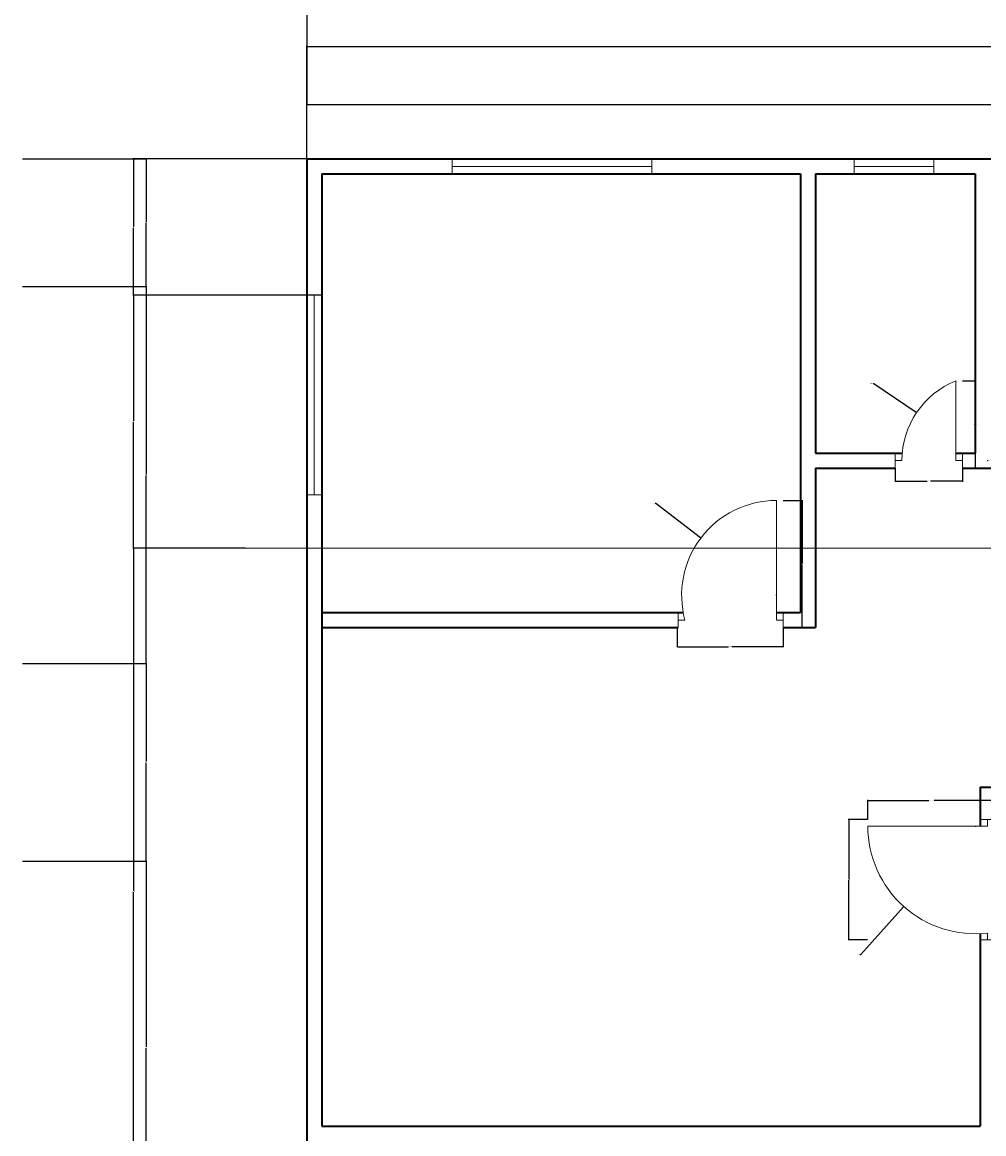
# Model space of a CAD drawing. Units: inches. Extents: x 992 to 2287, y 1476 to 2866.
# Tile 6 of 9: x 1531 to 1821, y 1987 to 2321. Entities that reach past the tile are written whole.
import ezdxf

# ---------------------------------------------------------------- set-up
doc = ezdxf.new("R2010")
doc.units = ezdxf.units.IN
for name, color, linetype, lineweight in [('A-ANNO-DIMS', 2, 'Continuous', 18), ('A-ANNO-SYMB', 2, 'Continuous', 18), ('A-DOOR', 3, 'Continuous', 18), ('A-GLAZ', 4, 'Continuous', 18), ('A-WALL', 7, 'Continuous', 35)]:
    doc.layers.add(name, color=color, linetype=linetype, lineweight=lineweight)
doc.styles.get("Standard").update_dxf_attribs({"font": 'arial.ttf'})
doc.dimstyles.get("Standard").update_dxf_attribs({"dimtxt": 0.18, "dimasz": 0.18, "dimexe": 0.18, "dimexo": 0.0625, "dimgap": 0.09, "dimtad": 0, "dimtih": 1, "dimtoh": 1, "dimdec": 4, "dimzin": 0, "dimdsep": 46, "dimtxsty": 'Standard', "dimcen": 0.09, "dimadec": 0, "dimazin": 0, "dimtfac": 1, "dimtdec": 4, "dimtofl": 0, "dimtmove": 0, "dimatfit": 3, "dimfxl": 1, "dimtolj": 1, "dimtzin": 0, "dimarcsym": 0})

# ---------------------------------------------------------------- blocks, each defined once
blk = doc.blocks.new('DOOR-SINGLE-36IN-01')
for p, q in [((36, 34.15), (0, 34.15)), ((38.25, 36.15), (33.75, 36.15)), ((33.75, 36.15), (36, 36.15)), ((36, 36.15), (36, 34.15)), ((33.75, 0), (38.25, 0)), ((36, 0), (36, 2)), ((38.25, 0), (36, 0))]:
    blk.add_line(p, q)
blk.add_arc((32.36, 34.15), 32.36, 180, 276.4675)
blk = doc.blocks.new('DOOR-SINGLE-24IN-04')
for p, q in [((18.2, 2.25), (18.2, 26.25)), ((0, 4.5), (0, 0)), ((20.2, 4.5), (20.2, 0)), ((0, 0), (0, 2.25)), ((0, 2.25), (2, 2.25)), ((20.2, 2.25), (18.2, 2.25)), ((20.2, 0), (20.2, 2.25))]:
    blk.add_line(p, q)
blk.add_arc((27.88, 2.25), 25.88, 111.9643, 180)
blk = doc.blocks.new('DOOR-SINGLE-36IN-06')
for p, q in [((29.52, 2.25), (29.52, 38.25)), ((0, 4.5), (0, 0)), ((31.52, 4.5), (31.52, 0)), ((0, 0), (0, 2.25)), ((0, 2.25), (2, 2.25)), ((31.52, 2.25), (29.52, 2.25)), ((31.52, 0), (31.52, 2.25))]:
    blk.add_line(p, q)
blk.add_arc((29.52, 9.74), 28.51, 90, 195.2187)
blk = doc.blocks.new('WINDOW-24IN-A')
for p, q in [((0, 24), (4.5, 24)), ((4.5, 24), (2.25, 24)), ((2.25, 24), (2.25, 0)), ((2.25, 0), (0, 0)), ((0, 0), (4.5, 0))]:
    blk.add_line(p, q)
blk = doc.blocks.new('WINDOW-60IN-A')
for p, q in [((4.5, 60), (0, 60)), ((0, 60), (2.25, 60)), ((2.25, 60), (2.25, 0)), ((2.25, 0), (0, 0)), ((0, 0), (4.5, 0))]:
    blk.add_line(p, q)
blk = doc.blocks.new('WINDOW-60IN-B')
for p, q in [((0, 4.5), (0, 0)), ((60, 2.25), (60, 4.5)), ((60, 4.5), (60, 0)), ((0, 0), (0, 2.25)), ((0, 2.25), (60, 2.25))]:
    blk.add_line(p, q)
blk = doc.blocks.new('*D49')
at = {"layer": 'A-ANNO-DIMS', "color": 0, "lineweight": -2, "transparency": 16777216}
for p, q in [((1785.64, 2081.37), (1785.64, 2087.23)), ((1785.82, 2087.05), (1803.98, 2087.05)), ((1823.71, 2087.05), (1805.56, 2087.05)), ((1823.89, 2081.37), (1823.89, 2087.23))]:
    blk.add_line(p, q, dxfattribs=at)
at = {"layer": 'A-ANNO-DIMS', "color": 0, "transparency": 16777216}
for points in [[(1785.82, 2087.08), (1785.82, 2087.02), (1785.64, 2087.05)], [(1823.71, 2087.08), (1823.71, 2087.02), (1823.89, 2087.05)]]:
    blk.add_solid(points, dxfattribs=at)
at = {"layer": 'Defpoints', "color": 0, "transparency": 16777216}
for p in [(1823.89, 2087.05), (1785.64, 2081.31), (1823.89, 2081.31)]:
    blk.add_point(p, dxfattribs=at)
at = {"layer": 'A-ANNO-DIMS', "color": 0, "transparency": 16777216, "insert": (1804.77, 2087.05), "char_height": 0.18, "attachment_point": 5}
blk.add_mtext('\\A1;D01 38 TYP.', dxfattribs=at)
blk = doc.blocks.new('*D50')
at = {"layer": 'A-ANNO-DIMS', "color": 0, "lineweight": -2, "transparency": 16777216}
for p, q in [((1785.58, 2081.31), (1779.73, 2081.31)), ((1779.91, 2081.13), (1779.91, 2063.42)), ((1779.91, 2045.34), (1779.91, 2063.06)), ((1785.58, 2045.16), (1779.73, 2045.16))]:
    blk.add_line(p, q, dxfattribs=at)
at = {"layer": 'A-ANNO-DIMS', "color": 0, "transparency": 16777216}
for points in [[(1779.88, 2081.13), (1779.94, 2081.13), (1779.91, 2081.31)], [(1779.88, 2045.34), (1779.94, 2045.34), (1779.91, 2045.16)]]:
    blk.add_solid(points, dxfattribs=at)
at = {"layer": 'Defpoints', "color": 0, "transparency": 16777216}
for p in [(1779.91, 2081.31), (1785.64, 2081.31), (1785.64, 2045.16)]:
    blk.add_point(p, dxfattribs=at)
at = {"layer": 'A-ANNO-DIMS', "color": 0, "transparency": 16777216, "insert": (1779.91, 2063.24), "char_height": 0.18, "attachment_point": 5}
blk.add_mtext('\\A1;36 TYP.', dxfattribs=at)
blk = doc.blocks.new('*D55')
at = {"layer": 'A-ANNO-DIMS', "color": 0, "lineweight": -2, "transparency": 16777216}
for p, q in [((1814.16, 2213.29), (1818.21, 2213.29)), ((1818.03, 2213.11), (1818.03, 2200.35)), ((1818.03, 2187.22), (1818.03, 2199.99)), ((1814.16, 2187.04), (1818.21, 2187.04))]:
    blk.add_line(p, q, dxfattribs=at)
at = {"layer": 'A-ANNO-DIMS', "color": 0, "transparency": 16777216}
for points in [[(1818, 2213.11), (1818.06, 2213.11), (1818.03, 2213.29)], [(1818, 2187.22), (1818.06, 2187.22), (1818.03, 2187.04)]]:
    blk.add_solid(points, dxfattribs=at)
at = {"layer": 'Defpoints', "color": 0, "transparency": 16777216}
for p in [(1814.09, 2213.29), (1818.03, 2213.29), (1814.09, 2187.04)]:
    blk.add_point(p, dxfattribs=at)
at = {"layer": 'A-ANNO-DIMS', "color": 0, "transparency": 16777216, "insert": (1818.03, 2200.17), "char_height": 0.18, "attachment_point": 5}
blk.add_mtext('\\A1;D04 26 TYP.', dxfattribs=at)
blk = doc.blocks.new('*D56')
at = {"layer": 'A-ANNO-DIMS', "color": 0, "lineweight": -2, "transparency": 16777216}
for p, q in [((1793.89, 2186.98), (1793.89, 2182.93)), ((1814.09, 2186.98), (1814.09, 2182.93)), ((1794.07, 2183.11), (1803.46, 2183.11)), ((1813.91, 2183.11), (1804.52, 2183.11))]:
    blk.add_line(p, q, dxfattribs=at)
at = {"layer": 'A-ANNO-DIMS', "color": 0, "transparency": 16777216}
for points in [[(1794.07, 2183.14), (1794.07, 2183.08), (1793.89, 2183.11)], [(1813.91, 2183.14), (1813.91, 2183.08), (1814.09, 2183.11)]]:
    blk.add_solid(points, dxfattribs=at)
at = {"layer": 'Defpoints', "color": 0, "transparency": 16777216}
for p in [(1793.89, 2187.04), (1814.09, 2187.04), (1814.09, 2183.11)]:
    blk.add_point(p, dxfattribs=at)
at = {"layer": 'A-ANNO-DIMS', "color": 0, "transparency": 16777216, "insert": (1803.99, 2183.11), "char_height": 0.18, "attachment_point": 5}
blk.add_mtext('\\A1;20 TYP.', dxfattribs=at)
blk = doc.blocks.new('*D59')
at = {"layer": 'A-ANNO-DIMS', "color": 0, "lineweight": -2, "transparency": 16777216}
for p, q in [((1760.2, 2177.29), (1766.06, 2177.29)), ((1765.88, 2177.11), (1765.88, 2158.35)), ((1765.88, 2139.22), (1765.88, 2157.99)), ((1760.2, 2139.04), (1766.06, 2139.04))]:
    blk.add_line(p, q, dxfattribs=at)
at = {"layer": 'A-ANNO-DIMS', "color": 0, "transparency": 16777216}
for points in [[(1765.85, 2177.11), (1765.91, 2177.11), (1765.88, 2177.29)], [(1765.85, 2139.22), (1765.91, 2139.22), (1765.88, 2139.04)]]:
    blk.add_solid(points, dxfattribs=at)
at = {"layer": 'Defpoints', "color": 0, "transparency": 16777216}
for p in [(1760.14, 2177.29), (1765.88, 2177.29), (1760.14, 2139.04)]:
    blk.add_point(p, dxfattribs=at)
at = {"layer": 'A-ANNO-DIMS', "color": 0, "transparency": 16777216, "insert": (1765.88, 2158.17), "char_height": 0.18, "attachment_point": 5}
blk.add_mtext('\\A1;D06 38 TYP.', dxfattribs=at)
blk = doc.blocks.new('*D60')
at = {"layer": 'A-ANNO-DIMS', "color": 0, "lineweight": -2, "transparency": 16777216}
for p, q in [((1728.3, 2138.98), (1728.3, 2133.13)), ((1760.14, 2138.98), (1760.14, 2133.13)), ((1728.48, 2133.31), (1743.69, 2133.31)), ((1759.96, 2133.31), (1744.75, 2133.31))]:
    blk.add_line(p, q, dxfattribs=at)
at = {"layer": 'A-ANNO-DIMS', "color": 0, "transparency": 16777216}
for points in [[(1728.48, 2133.34), (1728.48, 2133.28), (1728.3, 2133.31)], [(1759.96, 2133.34), (1759.96, 2133.28), (1760.14, 2133.31)]]:
    blk.add_solid(points, dxfattribs=at)
at = {"layer": 'Defpoints', "color": 0, "transparency": 16777216}
for p in [(1728.3, 2139.04), (1760.14, 2139.04), (1760.14, 2133.31)]:
    blk.add_point(p, dxfattribs=at)
at = {"layer": 'A-ANNO-DIMS', "color": 0, "transparency": 16777216, "insert": (1744.22, 2133.31), "char_height": 0.18, "attachment_point": 5}
blk.add_mtext('\\A1;32 TYP.', dxfattribs=at)
blk = doc.blocks.new('*D111')
at = {"layer": 'A-ANNO-DIMS', "color": 0, "lineweight": -2, "transparency": 16777216}
for p, q in [((1616.89, 2280.11), (1616.89, 2314.02)), ((1617.07, 2313.84), (1831.75, 2313.84)), ((2047.21, 2313.84), (1832.54, 2313.84)), ((2047.39, 2280.11), (2047.39, 2314.02))]:
    blk.add_line(p, q, dxfattribs=at)
at = {"layer": 'A-ANNO-DIMS', "color": 0, "transparency": 16777216}
for points in [[(1617.07, 2313.87), (1617.07, 2313.81), (1616.89, 2313.84)], [(2047.21, 2313.87), (2047.21, 2313.81), (2047.39, 2313.84)]]:
    blk.add_solid(points, dxfattribs=at)
at = {"layer": 'Defpoints', "color": 0, "transparency": 16777216}
for p in [(2047.39, 2313.84), (1616.89, 2280.04), (2047.39, 2280.04)]:
    blk.add_point(p, dxfattribs=at)
at = {"layer": 'A-ANNO-DIMS', "color": 0, "transparency": 16777216, "insert": (1832.14, 2313.84), "char_height": 0.18, "attachment_point": 5}
blk.add_mtext('\\A1;430.5', dxfattribs=at)
blk = doc.blocks.new('*D121')
at = {"layer": 'A-ANNO-DIMS', "color": 0, "lineweight": -2, "transparency": 16777216}
for p, q in [((1616.83, 2280.04), (1564.58, 2280.04)), ((1564.76, 2279.86), (1564.76, 2259.7)), ((1564.76, 2239.18), (1564.76, 2259.34)), ((1621.33, 2239), (1564.58, 2239))]:
    blk.add_line(p, q, dxfattribs=at)
at = {"layer": 'A-ANNO-DIMS', "color": 0, "transparency": 16777216}
for points in [[(1564.73, 2279.86), (1564.79, 2279.86), (1564.76, 2280.04)], [(1564.73, 2239.18), (1564.79, 2239.18), (1564.76, 2239)]]:
    blk.add_solid(points, dxfattribs=at)
at = {"layer": 'Defpoints', "color": 0, "transparency": 16777216}
for p in [(1564.76, 2280.04), (1616.89, 2280.04), (1621.39, 2239)]:
    blk.add_point(p, dxfattribs=at)
at = {"layer": 'A-ANNO-DIMS', "color": 0, "transparency": 16777216, "insert": (1564.76, 2259.52), "char_height": 0.18, "attachment_point": 5}
blk.add_mtext('\\A1;41.04', dxfattribs=at)
blk = doc.blocks.new('*D122')
at = {"layer": 'A-ANNO-DIMS', "color": 0, "lineweight": -2, "transparency": 16777216}
for p, q in [((1621.33, 2239), (1564.58, 2239)), ((1564.76, 2238.82), (1564.76, 2201.17)), ((1564.76, 2163.15), (1564.76, 2200.8)), ((1598.5, 2162.97), (1564.58, 2162.97))]:
    blk.add_line(p, q, dxfattribs=at)
at = {"layer": 'A-ANNO-DIMS', "color": 0, "transparency": 16777216}
for points in [[(1564.73, 2238.82), (1564.79, 2238.82), (1564.76, 2239)], [(1564.73, 2163.15), (1564.79, 2163.15), (1564.76, 2162.97)]]:
    blk.add_solid(points, dxfattribs=at)
at = {"layer": 'Defpoints', "color": 0, "transparency": 16777216}
for p in [(1564.76, 2239), (1621.39, 2239), (1598.56, 2162.97)]:
    blk.add_point(p, dxfattribs=at)
at = {"layer": 'A-ANNO-DIMS', "color": 0, "transparency": 16777216, "insert": (1564.76, 2200.99), "char_height": 0.18, "attachment_point": 5}
blk.add_mtext('\\A1;76.03', dxfattribs=at)
blk = doc.blocks.new('*D123')
at = {"layer": 'A-ANNO-DIMS', "color": 0, "lineweight": -2, "transparency": 16777216}
for p, q in [((1598.5, 2162.97), (1564.58, 2162.97)), ((1564.76, 2162.79), (1564.76, 2059.87)), ((1564.76, 1956.59), (1564.76, 2059.51)), ((1616.83, 1956.41), (1564.58, 1956.41))]:
    blk.add_line(p, q, dxfattribs=at)
at = {"layer": 'A-ANNO-DIMS', "color": 0, "transparency": 16777216}
for points in [[(1564.73, 2162.79), (1564.79, 2162.79), (1564.76, 2162.97)], [(1564.73, 1956.59), (1564.79, 1956.59), (1564.76, 1956.41)]]:
    blk.add_solid(points, dxfattribs=at)
at = {"layer": 'Defpoints', "color": 0, "transparency": 16777216}
for p in [(1564.76, 2162.97), (1598.56, 2162.97), (1616.89, 1956.41)]:
    blk.add_point(p, dxfattribs=at)
at = {"layer": 'A-ANNO-DIMS', "color": 0, "transparency": 16777216, "insert": (1564.76, 2059.69), "char_height": 0.18, "attachment_point": 5}
blk.add_mtext('\\A1;206.56', dxfattribs=at)
blk = doc.blocks.new('*D126')
at = {"layer": 'A-ANNO-DIMS', "color": 0, "lineweight": -2, "transparency": 16777216}
for p, q in [((1531.36, 2280.04), (1568.77, 2280.04)), ((1568.59, 2279.86), (1568.59, 2261.02)), ((1568.59, 2241.81), (1568.59, 2260.66)), ((1531.36, 2241.63), (1568.77, 2241.63))]:
    blk.add_line(p, q, dxfattribs=at)
at = {"layer": 'A-ANNO-DIMS', "color": 0, "transparency": 16777216}
for points in [[(1568.56, 2279.86), (1568.62, 2279.86), (1568.59, 2280.04)], [(1568.56, 2241.81), (1568.62, 2241.81), (1568.59, 2241.63)]]:
    blk.add_solid(points, dxfattribs=at)
at = {"layer": 'Defpoints', "color": 0, "transparency": 16777216}
for p in [(1531.29, 2280.04), (1568.59, 2280.04), (1531.29, 2241.63)]:
    blk.add_point(p, dxfattribs=at)
at = {"layer": 'A-ANNO-DIMS', "color": 0, "transparency": 16777216, "insert": (1568.59, 2260.84), "char_height": 0.18, "attachment_point": 5}
blk.add_mtext('\\A1;38.41', dxfattribs=at)
blk = doc.blocks.new('*D127')
at = {"layer": 'A-ANNO-DIMS', "color": 0, "lineweight": -2, "transparency": 16777216}
for p, q in [((1531.36, 2241.63), (1568.77, 2241.63)), ((1568.59, 2241.45), (1568.59, 2185.15)), ((1568.59, 2128.48), (1568.59, 2184.79)), ((1531.36, 2128.3), (1568.77, 2128.3))]:
    blk.add_line(p, q, dxfattribs=at)
at = {"layer": 'A-ANNO-DIMS', "color": 0, "transparency": 16777216}
for points in [[(1568.56, 2241.45), (1568.62, 2241.45), (1568.59, 2241.63)], [(1568.56, 2128.48), (1568.62, 2128.48), (1568.59, 2128.3)]]:
    blk.add_solid(points, dxfattribs=at)
at = {"layer": 'Defpoints', "color": 0, "transparency": 16777216}
for p in [(1531.29, 2241.63), (1568.59, 2241.63), (1531.29, 2128.3)]:
    blk.add_point(p, dxfattribs=at)
at = {"layer": 'A-ANNO-DIMS', "color": 0, "transparency": 16777216, "insert": (1568.59, 2184.97), "char_height": 0.18, "attachment_point": 5}
blk.add_mtext('\\A1;113.33', dxfattribs=at)
blk = doc.blocks.new('*D128')
at = {"layer": 'A-ANNO-DIMS', "color": 0, "lineweight": -2, "transparency": 16777216}
for p, q in [((1531.36, 2128.3), (1568.77, 2128.3)), ((1568.59, 2128.12), (1568.59, 2098.73)), ((1568.59, 2068.97), (1568.59, 2098.36)), ((1531.36, 2068.79), (1568.77, 2068.79))]:
    blk.add_line(p, q, dxfattribs=at)
at = {"layer": 'A-ANNO-DIMS', "color": 0, "transparency": 16777216}
for points in [[(1568.56, 2128.12), (1568.62, 2128.12), (1568.59, 2128.3)], [(1568.56, 2068.97), (1568.62, 2068.97), (1568.59, 2068.79)]]:
    blk.add_solid(points, dxfattribs=at)
at = {"layer": 'Defpoints', "color": 0, "transparency": 16777216}
for p in [(1531.29, 2128.3), (1568.59, 2128.3), (1531.29, 2068.79)]:
    blk.add_point(p, dxfattribs=at)
at = {"layer": 'A-ANNO-DIMS', "color": 0, "transparency": 16777216, "insert": (1568.59, 2098.54), "char_height": 0.18, "attachment_point": 5}
blk.add_mtext('\\A1;59.52', dxfattribs=at)
blk = doc.blocks.new('*D129')
at = {"layer": 'A-ANNO-DIMS', "color": 0, "lineweight": -2, "transparency": 16777216}
for p, q in [((1531.36, 2068.79), (1568.77, 2068.79)), ((1568.59, 2068.61), (1568.59, 2012.93)), ((1568.59, 1956.88), (1568.59, 2012.56)), ((1531.36, 1956.7), (1568.77, 1956.7))]:
    blk.add_line(p, q, dxfattribs=at)
at = {"layer": 'A-ANNO-DIMS', "color": 0, "transparency": 16777216}
for points in [[(1568.56, 2068.61), (1568.62, 2068.61), (1568.59, 2068.79)], [(1568.56, 1956.88), (1568.62, 1956.88), (1568.59, 1956.7)]]:
    blk.add_solid(points, dxfattribs=at)
at = {"layer": 'Defpoints', "color": 0, "transparency": 16777216}
for p in [(1531.29, 2068.79), (1568.59, 2068.79), (1531.29, 1956.7)]:
    blk.add_point(p, dxfattribs=at)
at = {"layer": 'A-ANNO-DIMS', "color": 0, "transparency": 16777216, "insert": (1568.59, 2012.74), "char_height": 0.18, "attachment_point": 5}
blk.add_mtext('\\A1;112.09', dxfattribs=at)
blk = doc.blocks.new('*D142')
at = {"layer": 'A-ANNO-DIMS', "color": 0, "lineweight": -2, "transparency": 16777216}
for p, q in [((1616.89, 2366.07), (1616.89, 2296.22)), ((2047.39, 2366.07), (2047.39, 2296.22)), ((1617.07, 2296.4), (1831.75, 2296.4)), ((2047.21, 2296.4), (1832.54, 2296.4))]:
    blk.add_line(p, q, dxfattribs=at)
at = {"layer": 'A-ANNO-DIMS', "color": 0, "transparency": 16777216}
for points in [[(1617.07, 2296.43), (1617.07, 2296.37), (1616.89, 2296.4)], [(2047.21, 2296.43), (2047.21, 2296.37), (2047.39, 2296.4)]]:
    blk.add_solid(points, dxfattribs=at)
at = {"layer": 'Defpoints', "color": 0, "transparency": 16777216}
for p in [(1616.89, 2366.13), (2047.39, 2366.13), (2047.39, 2296.4)]:
    blk.add_point(p, dxfattribs=at)
at = {"layer": 'A-ANNO-DIMS', "color": 0, "transparency": 16777216, "insert": (1832.14, 2296.4), "char_height": 0.18, "attachment_point": 5}
blk.add_mtext('\\A1;430.5', dxfattribs=at)
blk = doc.blocks.new('*D153')
at = {"layer": 'A-ANNO-DIMS', "color": 0, "lineweight": -2, "transparency": 16777216}
for p, q in [((1817.91, 2079.31), (1818.09, 2079.31)), ((1818, 2079.22), (1818, 2079.4)), ((1783.52, 2040.7), (1796.33, 2055.04)), ((1783.34, 2040.7), (1783.52, 2040.7))]:
    blk.add_line(p, q, dxfattribs=at)
at = {"layer": 'A-ANNO-DIMS', "color": 0, "transparency": 16777216}
blk.add_solid([(1796.31, 2055.06), (1796.35, 2055.02), (1796.45, 2055.18)], dxfattribs=at)
at = {"layer": 'Defpoints', "color": 0, "transparency": 16777216}
for p in [(1818, 2079.31), (1796.45, 2055.18)]:
    blk.add_point(p, dxfattribs=at)
at = {"layer": 'A-ANNO-DIMS', "color": 0, "transparency": 16777216, "insert": (1782.79, 2040.7), "char_height": 0.18, "attachment_point": 5}
blk.add_mtext('\\A1;R32.355', dxfattribs=at)
blk = doc.blocks.new('*D156')
at = {"layer": 'A-ANNO-DIMS', "color": 0, "lineweight": -2, "transparency": 16777216}
for p, q in [((1721.71, 2176.48), (1721.89, 2176.48)), ((1721.89, 2176.48), (1735.34, 2166.2)), ((1758.05, 2148.78), (1758.23, 2148.78)), ((1758.14, 2148.69), (1758.14, 2148.87))]:
    blk.add_line(p, q, dxfattribs=at)
at = {"layer": 'A-ANNO-DIMS', "color": 0, "transparency": 16777216}
blk.add_solid([(1735.36, 2166.23), (1735.33, 2166.18), (1735.49, 2166.09)], dxfattribs=at)
at = {"layer": 'Defpoints', "color": 0, "transparency": 16777216}
for p in [(1735.49, 2166.09), (1758.14, 2148.78)]:
    blk.add_point(p, dxfattribs=at)
at = {"layer": 'A-ANNO-DIMS', "color": 0, "transparency": 16777216, "insert": (1721.16, 2176.48), "char_height": 0.18, "attachment_point": 5}
blk.add_mtext('\\A1;R28.515', dxfattribs=at)
blk = doc.blocks.new('*D158')
at = {"layer": 'A-ANNO-DIMS', "color": 0, "lineweight": -2, "transparency": 16777216}
for p, q in [((1787.27, 2212.46), (1787.45, 2212.46)), ((1787.45, 2212.46), (1800.17, 2203.87)), ((1821.68, 2189.29), (1821.86, 2189.29)), ((1821.77, 2189.2), (1821.77, 2189.38))]:
    blk.add_line(p, q, dxfattribs=at)
at = {"layer": 'A-ANNO-DIMS', "color": 0, "transparency": 16777216}
blk.add_solid([(1800.19, 2203.9), (1800.16, 2203.85), (1800.32, 2203.77)], dxfattribs=at)
at = {"layer": 'Defpoints', "color": 0, "transparency": 16777216}
for p in [(1800.32, 2203.77), (1821.77, 2189.29)]:
    blk.add_point(p, dxfattribs=at)
at = {"layer": 'A-ANNO-DIMS', "color": 0, "transparency": 16777216, "insert": (1786.79, 2212.46), "char_height": 0.18, "attachment_point": 5}
blk.add_mtext('\\A1;R25.88', dxfattribs=at)

msp = doc.modelspace()

# ---------------------------------------------------------------- linework, layer by layer
at = {"layer": 'A-ANNO-SYMB'}
msp.add_line((1598.561, 2162.9718), (2084.6292, 2162.9718), dxfattribs=at)
at = {"layer": 'A-WALL'}
for p, q in [((1616.8946, 2280.0428), (2047.3946, 2280.0428)), ((1616.8946, 2280.0428), (2047.3946, 2280.0428)), ((1616.8946, 2280.0428), (1616.8946, 1677.0428)), ((1621.3946, 2275.5428), (1765.3946, 2275.5428)), ((1621.3946, 2275.5428), (1621.3946, 1989.0428)), ((1765.3946, 2275.5428), (1765.3946, 2143.5428)), ((1769.8946, 2275.5428), (1817.8946, 2275.5428)), ((1769.8946, 2275.5428), (1769.8946, 2191.5428)), ((1817.8946, 2275.5428), (1817.8946, 2191.5428)), ((1769.8946, 2191.5428), (1795.9926, 2191.5428)), ((1812.0937, 2191.5428), (1817.8946, 2191.5428)), ((1769.8946, 2187.0428), (1793.8946, 2187.0428)), ((1769.8946, 2187.0428), (1769.8946, 2139.0428)), ((1814.0937, 2187.0428), (1817.8946, 2187.0428)), ((1817.8946, 2187.0428), (1826.4319, 2187.0428)), ((1621.3946, 2143.5428), (1730.1121, 2143.5428)), ((1758.1422, 2143.5428), (1765.3946, 2143.5428)), ((1621.3946, 2139.0428), (1728.6274, 2139.0428)), ((1760.1422, 2139.0428), (1769.8946, 2139.0428)), ((1819.3946, 2091.0428), (2042.8946, 2091.0428)), ((1819.3946, 2091.0428), (1819.3946, 2079.3118)), ((1819.3946, 2046.9864), (1819.3946, 1989.0428)), ((1621.3946, 1989.0428), (1819.3946, 1989.0428))]:
    msp.add_line(p, q, dxfattribs=at)

# ---------------------------------------------------------------- block references
at = {"layer": 'A-DOOR'}
for name, p in [('DOOR-SINGLE-24IN-04', (1793.895, 2187.043)), ('DOOR-SINGLE-36IN-06', (1728.627, 2139.043)), ('DOOR-SINGLE-36IN-01', (1785.645, 2045.162))]:
    msp.add_blockref(name, p, dxfattribs=at)
at = {"layer": 'A-GLAZ'}
msp.add_blockref('WINDOW-60IN-B', (1660.6547, 2275.543), dxfattribs=at)
at = {"layer": 'A-GLAZ', "extrusion": (0, 0, -1), "zscale": -1, "rotation": 90}
msp.add_blockref('WINDOW-24IN-A', (-1781.5495, 2275.5432), dxfattribs=at)
at = {"layer": 'A-GLAZ', "rotation": 180}
msp.add_blockref('WINDOW-60IN-A', (1621.3941, 2239.0001), dxfattribs=at)

# ---------------------------------------------------------------- dimensions: what is measured, and where the dimension line sits
at = {"layer": 'A-ANNO-DIMS'}
for base, p1, p2, picture, middle in [((2047.3946, 2296.4015), (1616.8946, 2366.1302), (2047.3946, 2366.1302), '*D142', (1832.1446, 2296.4015)), ((2047.3946, 2313.8428), (1616.8946, 2280.0428), (2047.3946, 2280.0428), '*D111', (1832.1446, 2313.8428))]:
    dim = msp.add_linear_dim(base=base, p1=p1, p2=p2, dimstyle='Standard', override={"dimdec": 1, "dimlfac": 1, "dimrnd": 0, "dimzin": 0, "dimdsep": 46, "dimlunit": 2}, dxfattribs=at)
    dim.commit()
    dim.dimension.update_dxf_attribs({"geometry": picture, "text_midpoint": middle})
for base, p1, p2, picture, middle in [((1568.5936, 2280.0428), (1531.2936, 2241.633), (1531.2936, 2280.0428), '*D126', (1568.5936, 2260.8379)), ((1564.761, 2280.0428), (1621.3946, 2239.0001), (1616.8946, 2280.0428), '*D121', (1564.761, 2259.5214)), ((1568.5936, 2241.633), (1531.2936, 2128.3027), (1531.2936, 2241.633), '*D127', (1568.5936, 2184.9678)), ((1564.761, 2239.0001), (1598.561, 2162.9718), (1621.3946, 2239.0001), '*D122', (1564.761, 2200.986)), ((1564.761, 2162.9718), (1616.8946, 1956.4076), (1598.561, 2162.9718), '*D123', (1564.761, 2059.6897)), ((1568.5936, 2128.3027), (1531.2936, 2068.7863), (1531.2936, 2128.3027), '*D128', (1568.5936, 2098.5445)), ((1568.5936, 2068.7863), (1531.2936, 1956.7011), (1531.2936, 2068.7863), '*D129', (1568.5936, 2012.7437))]:
    dim = msp.add_linear_dim(base=base, p1=p1, p2=p2, angle=90, dimstyle='Standard', override={"dimdec": 2, "dimlfac": 1, "dimrnd": 0, "dimzin": 0, "dimdsep": 46, "dimlunit": 2}, dxfattribs=at)
    dim.commit()
    dim.dimension.update_dxf_attribs({"geometry": picture, "text_midpoint": middle})
for center, mpoint, override, picture, middle in [((1821.7729, 2189.2928), (1800.323, 2203.77), {"dimdec": 2, "dimlfac": 1, "dimrnd": 0, "dimzin": 0, "dimdsep": 46, "dimlunit": 2}, '*D158', (1786.7931, 2212.4563)), ((1758.1422, 2148.778), (1735.4871, 2166.0939), {"dimdec": 3, "dimlfac": 1, "dimrnd": 0, "dimzin": 0, "dimdsep": 46, "dimlunit": 2}, '*D156', (1721.1636, 2176.4834)), ((1818.0001, 2079.3118), (1796.4481, 2055.1791), {"dimdec": 3, "dimlfac": 1, "dimrnd": 0, "dimzin": 0, "dimdsep": 46, "dimlunit": 2}, '*D153', (1782.7864, 2040.6994))]:
    dim = msp.add_radius_dim(center=center, mpoint=mpoint, dimstyle='Standard', override=override, dxfattribs=at)
    dim.commit()
    dim.dimension.update_dxf_attribs({"geometry": picture, "text_midpoint": middle, "dimtype": 164})
for base, p1, p2, text, picture, middle in [((1818.0312, 2213.2928), (1814.0937, 2187.0428), (1814.0937, 2213.2928), 'D04 <> TYP.', '*D55', (1818.0312, 2200.1678)), ((1765.8797, 2177.2928), (1760.1422, 2139.0428), (1760.1422, 2177.2928), 'D06 <> TYP.', '*D59', (1765.8797, 2158.1678)), ((1779.9071, 2081.3118), (1785.6446, 2045.1622), (1785.6446, 2081.3118), '<> TYP.', '*D50', (1779.9071, 2063.237))]:
    dim = msp.add_linear_dim(base=base, p1=p1, p2=p2, angle=90, text=text, dimstyle='Standard', override={"dimdec": 0, "dimlfac": 1, "dimrnd": 0, "dimzin": 0, "dimdsep": 46, "dimlunit": 2}, dxfattribs=at)
    dim.commit()
    dim.dimension.update_dxf_attribs({"geometry": picture, "text_midpoint": middle})
for base, p1, p2, text, picture, middle in [((1814.0937, 2183.1053), (1793.8946, 2187.0428), (1814.0937, 2187.0428), '<> TYP.', '*D56', (1803.9941, 2183.1053)), ((1760.1422, 2133.3053), (1728.2953, 2139.0428), (1760.1422, 2139.0428), '<> TYP.', '*D60', (1744.2187, 2133.3053)), ((1823.8946, 2087.0493), (1785.6446, 2081.3118), (1823.8946, 2081.3118), 'D01 <> TYP.', '*D49', (1804.7696, 2087.0493))]:
    dim = msp.add_linear_dim(base=base, p1=p1, p2=p2, text=text, dimstyle='Standard', override={"dimdec": 0, "dimlfac": 1, "dimrnd": 0, "dimzin": 0, "dimdsep": 46, "dimlunit": 2}, dxfattribs=at)
    dim.commit()
    dim.dimension.update_dxf_attribs({"geometry": picture, "text_midpoint": middle})

doc.saveas('drawing.dxf')
